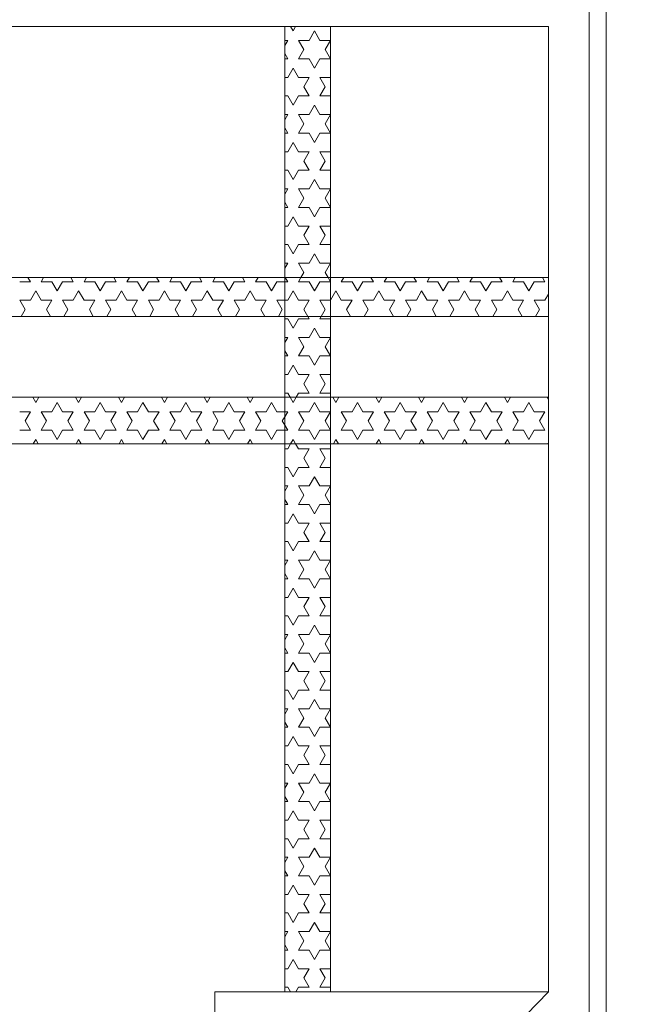
# Model space of a CAD drawing. Units: inches. Extents: x 1291 to 2095, y 532 to 1090.
# Tile 7 of 14: x 1640 to 1663, y 761 to 798. Entities that reach past the tile are written whole.
import ezdxf

# ---------------------------------------------------------------- set-up
doc = ezdxf.new("R2010")
doc.units = ezdxf.units.IN
doc.header["$MEASUREMENT"] = 0
doc.layers.add('A-ANNO-DIMS', color=2, linetype='Continuous', lineweight=18)
doc.layers.add('A-FURN', color=8, linetype='Continuous', lineweight=18)
doc.styles.get("Standard").update_dxf_attribs({"font": 'arial.ttf'})
doc.dimstyles.get("Standard").update_dxf_attribs({"dimtxt": 4, "dimasz": 0.18, "dimexe": 0.18, "dimexo": 0.0625, "dimgap": 0.09, "dimtad": 0, "dimtih": 1, "dimtoh": 1, "dimdec": 0, "dimrnd": 6, "dimzin": 0, "dimdsep": 46, "dimlunit": 3, "dimtxsty": 'Standard', "dimcen": 0.09, "dimadec": 0, "dimazin": 0, "dimtfac": 1, "dimtdec": 0, "dimtofl": 0, "dimtmove": 0, "dimatfit": 3, "dimfxl": 1, "dimtolj": 1, "dimtzin": 0, "dimarcsym": 0})

# ---------------------------------------------------------------- blocks, each defined once
blk = doc.blocks.new('A$C73B76B3A')
for p, q in [((0, 0), (0, 2)), ((0.02, 0.02), (0.02, 1.98)), ((0.4562, 1.5889), (0.0673, 1.1899)), ((0.4562, 1.5889), (0.4562, 1.1899)), ((0.4562, 1.1899), (0.0673, 1.1899)), ((0.0673, 1.1899), (0.0673, 0.0644)), ((0.3214, 1.1899), (0.3214, 0.0644)), ((0.3214, 1.1845), (0.3339, 1.1845)), ((0.3277, 1.1737), (0.3339, 1.1845)), ((0.3464, 1.1845), (0.3589, 1.1845)), ((0.3527, 1.1737), (0.3464, 1.1845)), ((0.3589, 1.1845), (0.362, 1.1899)), ((0.3714, 1.1845), (0.3683, 1.1899)), ((0.3714, 1.1845), (0.3749, 1.1845)), ((0.3749, 1.1899), (0.3749, 0.0644)), ((0.3339, 1.1629), (0.3277, 1.1737)), ((0.3464, 1.1629), (0.3527, 1.1737)), ((0.3214, 1.1629), (0.3339, 1.1629)), ((0.3464, 1.1629), (0.3589, 1.1629)), ((0.3652, 1.1521), (0.3589, 1.1629)), ((0.3652, 1.1521), (0.3714, 1.1629)), ((0.3714, 1.1629), (0.3749, 1.1629)), ((0.3339, 1.1412), (0.3402, 1.1521)), ((0.3464, 1.1412), (0.3402, 1.1521)), ((0.3214, 1.1412), (0.3339, 1.1412)), ((0.3277, 1.1304), (0.3214, 1.1412)), ((0.3464, 1.1412), (0.3589, 1.1412)), ((0.3527, 1.1304), (0.3589, 1.1412)), ((0.3714, 1.1412), (0.3749, 1.1412)), ((0.3749, 1.1352), (0.3714, 1.1412)), ((0.3214, 1.1196), (0.3277, 1.1304)), ((0.3589, 1.1196), (0.3527, 1.1304)), ((0.3714, 1.1196), (0.3749, 1.1257)), ((0.3214, 1.1196), (0.3339, 1.1196)), ((0.3402, 1.1088), (0.3339, 1.1196)), ((0.3402, 1.1088), (0.3464, 1.1196)), ((0.3464, 1.1196), (0.3589, 1.1196)), ((0.3714, 1.1196), (0.3749, 1.1196)), ((0.3589, 1.0979), (0.3652, 1.1088)), ((0.3714, 1.0979), (0.3652, 1.1088)), ((0.3214, 1.0979), (0.3339, 1.0979)), ((0.3277, 1.0871), (0.3339, 1.0979)), ((0.3464, 1.0979), (0.3589, 1.0979)), ((0.3527, 1.0871), (0.3464, 1.0979)), ((0.3714, 1.0979), (0.3749, 1.0979)), ((0.3339, 1.0763), (0.3277, 1.0871)), ((0.3464, 1.0763), (0.3527, 1.0871)), ((0.3214, 1.0763), (0.3339, 1.0763)), ((0.3464, 1.0763), (0.3589, 1.0763)), ((0.3652, 1.0655), (0.3589, 1.0763)), ((0.3652, 1.0655), (0.3714, 1.0763)), ((0.3714, 1.0763), (0.3749, 1.0763)), ((0.3339, 1.0546), (0.3402, 1.0655)), ((0.3464, 1.0546), (0.3402, 1.0655)), ((0.3214, 1.0546), (0.3339, 1.0546)), ((0.3277, 1.0438), (0.3214, 1.0546)), ((0.3464, 1.0546), (0.3589, 1.0546)), ((0.3527, 1.0438), (0.3589, 1.0546)), ((0.3714, 1.0546), (0.3749, 1.0546)), ((0.3749, 1.0486), (0.3714, 1.0546)), ((0.3214, 1.033), (0.3277, 1.0438)), ((0.3589, 1.033), (0.3527, 1.0438)), ((0.3714, 1.033), (0.3749, 1.0391)), ((0.3214, 1.033), (0.3339, 1.033)), ((0.3402, 1.0222), (0.3339, 1.033)), ((0.3402, 1.0222), (0.3464, 1.033)), ((0.3464, 1.033), (0.3589, 1.033)), ((0.3589, 1.0113), (0.3652, 1.0222)), ((0.3714, 1.0113), (0.3652, 1.0222)), ((0.3714, 1.033), (0.3749, 1.033)), ((0.3214, 1.0113), (0.3339, 1.0113)), ((0.3277, 1.0005), (0.3339, 1.0113)), ((0.3464, 1.0113), (0.3589, 1.0113)), ((0.3527, 1.0005), (0.3464, 1.0113)), ((0.3714, 1.0113), (0.3749, 1.0113)), ((0.3339, 0.9897), (0.3277, 1.0005)), ((0.3464, 0.9897), (0.3527, 1.0005)), ((0.3214, 0.9897), (0.3339, 0.9897)), ((0.3464, 0.9897), (0.3589, 0.9897)), ((0.3652, 0.9789), (0.3589, 0.9897)), ((0.3652, 0.9789), (0.3714, 0.9897)), ((0.3714, 0.9897), (0.3749, 0.9897)), ((0.3339, 0.968), (0.3402, 0.9789)), ((0.3464, 0.968), (0.3402, 0.9789)), ((0.3214, 0.968), (0.3339, 0.968)), ((0.3277, 0.9572), (0.3214, 0.968)), ((0.3464, 0.968), (0.3589, 0.968)), ((0.3527, 0.9572), (0.3589, 0.968)), ((0.3714, 0.968), (0.3749, 0.968)), ((0.3749, 0.962), (0.3714, 0.968)), ((0.3214, 0.9464), (0.3277, 0.9572)), ((0.3589, 0.9464), (0.3527, 0.9572)), ((0.3214, 0.9464), (0.3339, 0.9464)), ((0.3402, 0.9356), (0.3339, 0.9464)), ((0.3402, 0.9356), (0.3464, 0.9464)), ((0.3464, 0.9464), (0.3589, 0.9464)), ((0.3714, 0.9464), (0.3749, 0.9525)), ((0.3714, 0.9464), (0.3749, 0.9464)), ((0.3589, 0.9247), (0.3652, 0.9356)), ((0.3714, 0.9247), (0.3652, 0.9356)), ((0.3214, 0.9247), (0.3339, 0.9247)), ((0.3277, 0.9139), (0.3339, 0.9247)), ((0.3464, 0.9247), (0.3589, 0.9247)), ((0.3527, 0.9139), (0.3464, 0.9247)), ((0.3714, 0.9247), (0.3749, 0.9247)), ((0.3339, 0.9031), (0.3277, 0.9139)), ((0.3464, 0.9031), (0.3527, 0.9139)), ((0.3214, 0.9031), (0.3339, 0.9031)), ((0.3464, 0.9031), (0.3589, 0.9031)), ((0.3652, 0.8923), (0.3589, 0.9031)), ((0.3652, 0.8923), (0.3714, 0.9031)), ((0.3714, 0.9031), (0.3749, 0.9031)), ((0.3339, 0.8814), (0.3402, 0.8923)), ((0.3464, 0.8814), (0.3402, 0.8923)), ((0.3214, 0.8814), (0.3339, 0.8814)), ((0.3277, 0.8706), (0.3214, 0.8814)), ((0.3464, 0.8814), (0.3589, 0.8814)), ((0.3527, 0.8706), (0.3589, 0.8814)), ((0.3714, 0.8814), (0.3749, 0.8814)), ((0.3749, 0.8754), (0.3714, 0.8814)), ((0.3214, 0.8598), (0.3277, 0.8706)), ((0.3589, 0.8598), (0.3527, 0.8706)), ((0.3714, 0.8598), (0.3749, 0.8659)), ((0.3214, 0.8598), (0.3339, 0.8598)), ((0.3402, 0.849), (0.3339, 0.8598)), ((0.3402, 0.849), (0.3464, 0.8598)), ((0.3464, 0.8598), (0.3589, 0.8598)), ((0.3714, 0.8598), (0.3749, 0.8598)), ((0.3214, 0.8381), (0.3339, 0.8381)), ((0.3277, 0.8273), (0.3339, 0.8381)), ((0.3464, 0.8381), (0.3589, 0.8381)), ((0.3527, 0.8273), (0.3464, 0.8381)), ((0.3589, 0.8381), (0.3652, 0.849)), ((0.3714, 0.8381), (0.3652, 0.849)), ((0.3714, 0.8381), (0.3749, 0.8381)), ((0.3339, 0.8165), (0.3277, 0.8273)), ((0.3464, 0.8165), (0.3527, 0.8273)), ((0.3214, 0.8165), (0.3339, 0.8165)), ((0.3464, 0.8165), (0.3589, 0.8165)), ((0.3652, 0.8057), (0.3589, 0.8165)), ((0.3652, 0.8057), (0.3714, 0.8165)), ((0.3714, 0.8165), (0.3749, 0.8165)), ((0.3339, 0.7948), (0.3402, 0.8057)), ((0.3464, 0.7948), (0.3402, 0.8057)), ((0.3214, 0.7948), (0.3339, 0.7948)), ((0.3277, 0.784), (0.3214, 0.7948)), ((0.3464, 0.7948), (0.3589, 0.7948)), ((0.3527, 0.784), (0.3589, 0.7948)), ((0.3714, 0.7948), (0.3749, 0.7948)), ((0.3749, 0.7888), (0.3714, 0.7948)), ((0.3214, 0.7732), (0.3277, 0.784)), ((0.3589, 0.7732), (0.3527, 0.784)), ((0.3214, 0.7732), (0.3339, 0.7732)), ((0.3402, 0.7624), (0.3339, 0.7732)), ((0.3402, 0.7624), (0.3464, 0.7732)), ((0.3464, 0.7732), (0.3589, 0.7732)), ((0.3714, 0.7732), (0.3749, 0.7793)), ((0.3714, 0.7732), (0.3749, 0.7732)), ((0.3589, 0.7515), (0.3652, 0.7624)), ((0.3714, 0.7515), (0.3652, 0.7624)), ((0.3214, 0.7515), (0.3339, 0.7515)), ((0.3277, 0.7407), (0.3339, 0.7515)), ((0.3464, 0.7515), (0.3589, 0.7515)), ((0.3527, 0.7407), (0.3464, 0.7515)), ((0.3714, 0.7515), (0.3749, 0.7515)), ((0.3339, 0.7299), (0.3277, 0.7407)), ((0.3464, 0.7299), (0.3527, 0.7407)), ((0.3214, 0.7299), (0.3339, 0.7299)), ((0.3464, 0.7299), (0.3589, 0.7299)), ((0.3652, 0.7191), (0.3589, 0.7299)), ((0.3652, 0.7191), (0.3714, 0.7299)), ((0.3714, 0.7299), (0.3749, 0.7299)), ((0.3339, 0.7082), (0.3402, 0.7191)), ((0.3464, 0.7082), (0.3402, 0.7191)), ((0.3214, 0.7082), (0.3339, 0.7082)), ((0.3277, 0.6974), (0.3214, 0.7082)), ((0.3464, 0.7082), (0.3589, 0.7082)), ((0.3527, 0.6974), (0.3589, 0.7082)), ((0.3714, 0.7082), (0.3749, 0.7082)), ((0.3749, 0.7022), (0.3714, 0.7082)), ((0.3214, 0.6866), (0.3277, 0.6974)), ((0.3589, 0.6866), (0.3527, 0.6974)), ((0.3714, 0.6866), (0.3749, 0.6926)), ((0.3214, 0.6866), (0.3339, 0.6866)), ((0.3402, 0.6758), (0.3339, 0.6866)), ((0.3402, 0.6758), (0.3464, 0.6866)), ((0.3464, 0.6866), (0.3589, 0.6866)), ((0.3714, 0.6866), (0.3749, 0.6866)), ((0.3589, 0.6649), (0.3652, 0.6758)), ((0.3714, 0.6649), (0.3652, 0.6758)), ((0.3214, 0.6649), (0.3339, 0.6649)), ((0.3277, 0.6541), (0.3339, 0.6649)), ((0.3464, 0.6649), (0.3589, 0.6649)), ((0.3527, 0.6541), (0.3464, 0.6649)), ((0.3714, 0.6649), (0.3749, 0.6649)), ((0.3214, 0.6433), (0.3339, 0.6433)), ((0.3339, 0.6433), (0.3277, 0.6541)), ((0.3464, 0.6433), (0.3527, 0.6541)), ((0.3464, 0.6433), (0.3589, 0.6433)), ((0.3652, 0.6325), (0.3589, 0.6433)), ((0.3652, 0.6325), (0.3714, 0.6433)), ((0.3714, 0.6433), (0.3749, 0.6433)), ((0.3339, 0.6216), (0.3402, 0.6325)), ((0.3464, 0.6216), (0.3402, 0.6325)), ((0.3214, 0.6216), (0.3339, 0.6216)), ((0.3277, 0.6108), (0.3214, 0.6216)), ((0.3464, 0.6216), (0.3589, 0.6216)), ((0.3527, 0.6108), (0.3589, 0.6216)), ((0.3714, 0.6216), (0.3749, 0.6216)), ((0.3749, 0.6156), (0.3714, 0.6216)), ((0.3214, 0.6), (0.3277, 0.6108)), ((0.3589, 0.6), (0.3527, 0.6108)), ((0.3214, 0.6), (0.3339, 0.6)), ((0.3402, 0.5892), (0.3339, 0.6)), ((0.3402, 0.5892), (0.3464, 0.6)), ((0.3464, 0.6), (0.3589, 0.6)), ((0.3714, 0.6), (0.3749, 0.606)), ((0.3714, 0.6), (0.3749, 0.6)), ((0.3589, 0.5783), (0.3652, 0.5892)), ((0.3714, 0.5783), (0.3652, 0.5892)), ((0.3214, 0.5783), (0.3339, 0.5783)), ((0.3277, 0.5675), (0.3339, 0.5783)), ((0.3464, 0.5783), (0.3589, 0.5783)), ((0.3527, 0.5675), (0.3464, 0.5783)), ((0.3714, 0.5783), (0.3749, 0.5783)), ((0.3339, 0.5567), (0.3277, 0.5675)), ((0.3464, 0.5567), (0.3527, 0.5675)), ((0.3214, 0.5567), (0.3339, 0.5567)), ((0.3464, 0.5567), (0.3589, 0.5567)), ((0.3623, 0.5509), (0.3589, 0.5567)), ((0.3681, 0.5509), (0.3714, 0.5567)), ((0.3714, 0.5567), (0.3749, 0.5567)), ((1.2954, 0.5509), (0.0673, 0.5509)), ((0.0673, 0.5495), (0.0681, 0.5509)), ((0.0839, 0.535), (0.0902, 0.5459)), ((0.0964, 0.535), (0.0902, 0.5459)), ((0.1152, 0.5459), (0.1123, 0.5509)), ((0.1152, 0.5459), (0.1181, 0.5509)), ((0.1339, 0.535), (0.1402, 0.5459)), ((0.1464, 0.535), (0.1402, 0.5459)), ((0.1652, 0.5459), (0.1623, 0.5509)), ((0.1652, 0.5459), (0.1681, 0.5509)), ((0.1839, 0.535), (0.1902, 0.5459)), ((0.1964, 0.535), (0.1902, 0.5459)), ((0.2152, 0.5459), (0.2123, 0.5509)), ((0.2152, 0.5459), (0.2181, 0.5509)), ((0.2339, 0.535), (0.2402, 0.5459)), ((0.2464, 0.535), (0.2402, 0.5459)), ((0.2652, 0.5459), (0.2623, 0.5509)), ((0.2652, 0.5459), (0.2681, 0.5509)), ((0.2839, 0.535), (0.2902, 0.5459)), ((0.2964, 0.535), (0.2902, 0.5459)), ((0.3152, 0.5459), (0.3123, 0.5509)), ((0.3152, 0.5459), (0.3181, 0.5509)), ((0.3339, 0.535), (0.3402, 0.5459)), ((0.3464, 0.535), (0.3402, 0.5459)), ((0.3652, 0.5459), (0.3623, 0.5509)), ((0.3652, 0.5459), (0.3681, 0.5509)), ((0.3839, 0.535), (0.3902, 0.5459)), ((0.3964, 0.535), (0.3902, 0.5459)), ((0.4152, 0.5459), (0.4123, 0.5509)), ((0.4152, 0.5459), (0.4181, 0.5509)), ((0.4339, 0.535), (0.4402, 0.5459)), ((0.4464, 0.535), (0.4402, 0.5459)), ((0.4652, 0.5459), (0.4623, 0.5509)), ((0.4652, 0.5459), (0.4681, 0.5509)), ((0.4839, 0.535), (0.4902, 0.5459)), ((0.4964, 0.535), (0.4902, 0.5459)), ((0.5152, 0.5459), (0.5123, 0.5509)), ((0.5152, 0.5459), (0.5181, 0.5509)), ((0.5339, 0.535), (0.5402, 0.5459)), ((0.5464, 0.535), (0.5402, 0.5459)), ((0.5652, 0.5459), (0.5623, 0.5509)), ((0.5652, 0.5459), (0.5681, 0.5509)), ((0.5839, 0.535), (0.5902, 0.5459)), ((0.5964, 0.535), (0.5902, 0.5459)), ((0.6152, 0.5459), (0.6123, 0.5509)), ((0.6152, 0.5459), (0.6181, 0.5509)), ((0.6339, 0.535), (0.6402, 0.5459)), ((0.6464, 0.535), (0.6402, 0.5459)), ((0.6652, 0.5459), (0.6623, 0.5509)), ((0.6652, 0.5459), (0.6681, 0.5509)), ((0.0714, 0.535), (0.0839, 0.535)), ((0.0777, 0.5242), (0.0714, 0.535)), ((0.0964, 0.535), (0.1089, 0.535)), ((0.1027, 0.5242), (0.1089, 0.535)), ((0.1214, 0.535), (0.1339, 0.535)), ((0.1277, 0.5242), (0.1214, 0.535)), ((0.1464, 0.535), (0.1589, 0.535)), ((0.1527, 0.5242), (0.1589, 0.535)), ((0.1714, 0.535), (0.1839, 0.535)), ((0.1777, 0.5242), (0.1714, 0.535)), ((0.1964, 0.535), (0.2089, 0.535)), ((0.2027, 0.5242), (0.2089, 0.535)), ((0.2214, 0.535), (0.2339, 0.535)), ((0.2277, 0.5242), (0.2214, 0.535)), ((0.2464, 0.535), (0.2589, 0.535)), ((0.2527, 0.5242), (0.2589, 0.535)), ((0.2714, 0.535), (0.2839, 0.535)), ((0.2777, 0.5242), (0.2714, 0.535)), ((0.2964, 0.535), (0.3089, 0.535)), ((0.3027, 0.5242), (0.3089, 0.535)), ((0.3214, 0.535), (0.3214, 0.535)), ((0.3214, 0.535), (0.3339, 0.535)), ((0.3214, 0.535), (0.3214, 0.535)), ((0.3277, 0.5242), (0.3214, 0.535)), ((0.3464, 0.535), (0.3589, 0.535)), ((0.3527, 0.5242), (0.3589, 0.535)), ((0.3714, 0.535), (0.3749, 0.535)), ((0.3749, 0.529), (0.3714, 0.535)), ((0.3749, 0.535), (0.3839, 0.535)), ((0.3777, 0.5242), (0.3749, 0.529)), ((0.3964, 0.535), (0.4089, 0.535)), ((0.4027, 0.5242), (0.4089, 0.535)), ((0.4214, 0.535), (0.4339, 0.535)), ((0.4277, 0.5242), (0.4214, 0.535)), ((0.4464, 0.535), (0.4589, 0.535)), ((0.4527, 0.5242), (0.4589, 0.535)), ((0.4714, 0.535), (0.4839, 0.535)), ((0.4777, 0.5242), (0.4714, 0.535)), ((0.4964, 0.535), (0.5089, 0.535)), ((0.5027, 0.5242), (0.5089, 0.535)), ((0.5214, 0.535), (0.5339, 0.535)), ((0.5277, 0.5242), (0.5214, 0.535)), ((0.5464, 0.535), (0.5589, 0.535)), ((0.5527, 0.5242), (0.5589, 0.535)), ((0.5714, 0.535), (0.5839, 0.535)), ((0.5777, 0.5242), (0.5714, 0.535)), ((0.5964, 0.535), (0.6089, 0.535)), ((0.6027, 0.5242), (0.6089, 0.535)), ((0.6214, 0.535), (0.6339, 0.535)), ((0.6277, 0.5242), (0.6214, 0.535)), ((0.6464, 0.535), (0.6589, 0.535)), ((0.6527, 0.5242), (0.6589, 0.535)), ((0.6714, 0.535), (0.6839, 0.535)), ((0.6777, 0.5242), (0.6714, 0.535)), ((0.0714, 0.5134), (0.0777, 0.5242)), ((0.1089, 0.5134), (0.1027, 0.5242)), ((0.1214, 0.5134), (0.1277, 0.5242)), ((0.1589, 0.5134), (0.1527, 0.5242)), ((0.1714, 0.5134), (0.1777, 0.5242)), ((0.2089, 0.5134), (0.2027, 0.5242)), ((0.2214, 0.5134), (0.2277, 0.5242)), ((0.2589, 0.5134), (0.2527, 0.5242)), ((0.2714, 0.5134), (0.2777, 0.5242)), ((0.3089, 0.5134), (0.3027, 0.5242)), ((0.3214, 0.5134), (0.3277, 0.5242)), ((0.3589, 0.5134), (0.3527, 0.5242)), ((0.3714, 0.5134), (0.3749, 0.5194)), ((0.3749, 0.5194), (0.3777, 0.5242)), ((0.4089, 0.5134), (0.4027, 0.5242)), ((0.4214, 0.5134), (0.4277, 0.5242)), ((0.4589, 0.5134), (0.4527, 0.5242)), ((0.4714, 0.5134), (0.4777, 0.5242)), ((0.5089, 0.5134), (0.5027, 0.5242)), ((0.5214, 0.5134), (0.5277, 0.5242)), ((0.5589, 0.5134), (0.5527, 0.5242)), ((0.5714, 0.5134), (0.5777, 0.5242)), ((0.6089, 0.5134), (0.6027, 0.5242)), ((0.6214, 0.5134), (0.6277, 0.5242)), ((0.6589, 0.5134), (0.6527, 0.5242)), ((0.6714, 0.5134), (0.6777, 0.5242)), ((0.0714, 0.5134), (0.0839, 0.5134)), ((0.0902, 0.5026), (0.0839, 0.5134)), ((0.0902, 0.5026), (0.0964, 0.5134)), ((0.0964, 0.5134), (0.1089, 0.5134)), ((0.1214, 0.5134), (0.1339, 0.5134)), ((0.1402, 0.5026), (0.1339, 0.5134)), ((0.1402, 0.5026), (0.1464, 0.5134)), ((0.1464, 0.5134), (0.1589, 0.5134)), ((0.1714, 0.5134), (0.1839, 0.5134)), ((0.1902, 0.5026), (0.1839, 0.5134)), ((0.1902, 0.5026), (0.1964, 0.5134)), ((0.1964, 0.5134), (0.2089, 0.5134)), ((0.2214, 0.5134), (0.2339, 0.5134)), ((0.2402, 0.5026), (0.2339, 0.5134)), ((0.2402, 0.5026), (0.2464, 0.5134)), ((0.2464, 0.5134), (0.2589, 0.5134)), ((0.2714, 0.5134), (0.2839, 0.5134)), ((0.2902, 0.5026), (0.2839, 0.5134)), ((0.2902, 0.5026), (0.2964, 0.5134)), ((0.2964, 0.5134), (0.3089, 0.5134)), ((0.3214, 0.5134), (0.3214, 0.5134)), ((0.3214, 0.5134), (0.3339, 0.5134)), ((0.3214, 0.5134), (0.3214, 0.5134)), ((0.3402, 0.5026), (0.3339, 0.5134)), ((0.3402, 0.5026), (0.3464, 0.5134)), ((0.3464, 0.5134), (0.3589, 0.5134)), ((0.3714, 0.5134), (0.3749, 0.5134)), ((0.3749, 0.5134), (0.3839, 0.5134)), ((0.3902, 0.5026), (0.3839, 0.5134)), ((0.3902, 0.5026), (0.3964, 0.5134)), ((0.3964, 0.5134), (0.4089, 0.5134)), ((0.4214, 0.5134), (0.4339, 0.5134)), ((0.4402, 0.5026), (0.4339, 0.5134)), ((0.4402, 0.5026), (0.4464, 0.5134)), ((0.4464, 0.5134), (0.4589, 0.5134)), ((0.4714, 0.5134), (0.4839, 0.5134)), ((0.4902, 0.5026), (0.4839, 0.5134)), ((0.4902, 0.5026), (0.4964, 0.5134)), ((0.4964, 0.5134), (0.5089, 0.5134)), ((0.5214, 0.5134), (0.5339, 0.5134)), ((0.5402, 0.5026), (0.5339, 0.5134)), ((0.5402, 0.5026), (0.5464, 0.5134)), ((0.5464, 0.5134), (0.5589, 0.5134)), ((0.5714, 0.5134), (0.5839, 0.5134)), ((0.5902, 0.5026), (0.5839, 0.5134)), ((0.5902, 0.5026), (0.5964, 0.5134)), ((0.5964, 0.5134), (0.6089, 0.5134)), ((0.6214, 0.5134), (0.6339, 0.5134)), ((0.6402, 0.5026), (0.6339, 0.5134)), ((0.6402, 0.5026), (0.6464, 0.5134)), ((0.6464, 0.5134), (0.6589, 0.5134)), ((0.6714, 0.5134), (0.6839, 0.5134)), ((0.0687, 0.4965), (0.0673, 0.4989)), ((1.2954, 0.4965), (0.0673, 0.4965)), ((0.1117, 0.4965), (0.1152, 0.5026)), ((0.1187, 0.4965), (0.1152, 0.5026)), ((0.1617, 0.4965), (0.1652, 0.5026)), ((0.1687, 0.4965), (0.1652, 0.5026)), ((0.2117, 0.4965), (0.2152, 0.5026)), ((0.2187, 0.4965), (0.2152, 0.5026)), ((0.2617, 0.4965), (0.2652, 0.5026)), ((0.2687, 0.4965), (0.2652, 0.5026)), ((0.3117, 0.4965), (0.3152, 0.5026)), ((0.3187, 0.4965), (0.3152, 0.5026)), ((0.3589, 0.4917), (0.3617, 0.4965)), ((0.3617, 0.4965), (0.3652, 0.5026)), ((0.3687, 0.4965), (0.3652, 0.5026)), ((0.3714, 0.4917), (0.3687, 0.4965)), ((0.4117, 0.4965), (0.4152, 0.5026)), ((0.4187, 0.4965), (0.4152, 0.5026)), ((0.4617, 0.4965), (0.4652, 0.5026)), ((0.4687, 0.4965), (0.4652, 0.5026)), ((0.5117, 0.4965), (0.5152, 0.5026)), ((0.5187, 0.4965), (0.5152, 0.5026)), ((0.5617, 0.4965), (0.5652, 0.5026)), ((0.5687, 0.4965), (0.5652, 0.5026)), ((0.6117, 0.4965), (0.6152, 0.5026)), ((0.6187, 0.4965), (0.6152, 0.5026)), ((0.6617, 0.4965), (0.6652, 0.5026)), ((0.6687, 0.4965), (0.6652, 0.5026)), ((0.3214, 0.4917), (0.3339, 0.4917)), ((0.3277, 0.4809), (0.3339, 0.4917)), ((0.3464, 0.4917), (0.3589, 0.4917)), ((0.3527, 0.4809), (0.3464, 0.4917)), ((0.3714, 0.4917), (0.3749, 0.4917)), ((0.3339, 0.4701), (0.3277, 0.4809)), ((0.3464, 0.4701), (0.3527, 0.4809)), ((0.3214, 0.4701), (0.3339, 0.4701)), ((0.3339, 0.4484), (0.3402, 0.4593)), ((0.3464, 0.4484), (0.3402, 0.4593)), ((0.3464, 0.4701), (0.3589, 0.4701)), ((0.3652, 0.4593), (0.3589, 0.4701)), ((0.3652, 0.4593), (0.3714, 0.4701)), ((0.3714, 0.4701), (0.3749, 0.4701)), ((0.3214, 0.4484), (0.3339, 0.4484)), ((0.3277, 0.4376), (0.3214, 0.4484)), ((0.3464, 0.4484), (0.3589, 0.4484)), ((0.3527, 0.4376), (0.3589, 0.4484)), ((0.3714, 0.4484), (0.3749, 0.4484)), ((0.3749, 0.4424), (0.3714, 0.4484)), ((0.3214, 0.4268), (0.3277, 0.4376)), ((0.3589, 0.4268), (0.3527, 0.4376)), ((0.3214, 0.4268), (0.3339, 0.4268)), ((0.3402, 0.4159), (0.3339, 0.4268)), ((0.3402, 0.4159), (0.3464, 0.4268)), ((0.3464, 0.4268), (0.3589, 0.4268)), ((0.3714, 0.4268), (0.3749, 0.4328)), ((0.3714, 0.4268), (0.3749, 0.4268)), ((0.3589, 0.4051), (0.3652, 0.4159)), ((0.3714, 0.4051), (0.3652, 0.4159)), ((1.2954, 0.4023), (0.0673, 0.4023)), ((0.0777, 0.3943), (0.0823, 0.4023)), ((0.1027, 0.3943), (0.0981, 0.4023)), ((0.1277, 0.3943), (0.1323, 0.4023)), ((0.1527, 0.3943), (0.1481, 0.4023)), ((0.1777, 0.3943), (0.1823, 0.4023)), ((0.2027, 0.3943), (0.1981, 0.4023)), ((0.2277, 0.3943), (0.2323, 0.4023)), ((0.2527, 0.3943), (0.2481, 0.4023)), ((0.2777, 0.3943), (0.2823, 0.4023)), ((0.3027, 0.3943), (0.2981, 0.4023)), ((0.3214, 0.4051), (0.3339, 0.4051)), ((0.3277, 0.3943), (0.3323, 0.4023)), ((0.3323, 0.4023), (0.3339, 0.4051)), ((0.3464, 0.4051), (0.3589, 0.4051)), ((0.3481, 0.4023), (0.3464, 0.4051)), ((0.3527, 0.3943), (0.3481, 0.4023)), ((0.3714, 0.4051), (0.3749, 0.4051)), ((0.3777, 0.3943), (0.3823, 0.4023)), ((0.4027, 0.3943), (0.3981, 0.4023)), ((0.4277, 0.3943), (0.4323, 0.4023)), ((0.4527, 0.3943), (0.4481, 0.4023)), ((0.4777, 0.3943), (0.4823, 0.4023)), ((0.5027, 0.3943), (0.4981, 0.4023)), ((0.5277, 0.3943), (0.5323, 0.4023)), ((0.5527, 0.3943), (0.5481, 0.4023)), ((0.5777, 0.3943), (0.5823, 0.4023)), ((0.6027, 0.3943), (0.5981, 0.4023)), ((0.6277, 0.3943), (0.6323, 0.4023)), ((0.6527, 0.3943), (0.6481, 0.4023)), ((0.6777, 0.3943), (0.6823, 0.4023)), ((0.0839, 0.3835), (0.0777, 0.3943)), ((0.0964, 0.3835), (0.1027, 0.3943)), ((0.1339, 0.3835), (0.1277, 0.3943)), ((0.1464, 0.3835), (0.1527, 0.3943)), ((0.1839, 0.3835), (0.1777, 0.3943)), ((0.1964, 0.3835), (0.2027, 0.3943)), ((0.2339, 0.3835), (0.2277, 0.3943)), ((0.2464, 0.3835), (0.2527, 0.3943)), ((0.2839, 0.3835), (0.2777, 0.3943)), ((0.2964, 0.3835), (0.3027, 0.3943)), ((0.3339, 0.3835), (0.3277, 0.3943)), ((0.3464, 0.3835), (0.3527, 0.3943)), ((0.3839, 0.3835), (0.3777, 0.3943)), ((0.3964, 0.3835), (0.4027, 0.3943)), ((0.4339, 0.3835), (0.4277, 0.3943)), ((0.4464, 0.3835), (0.4527, 0.3943)), ((0.4839, 0.3835), (0.4777, 0.3943)), ((0.4964, 0.3835), (0.5027, 0.3943)), ((0.5339, 0.3835), (0.5277, 0.3943)), ((0.5464, 0.3835), (0.5527, 0.3943)), ((0.5839, 0.3835), (0.5777, 0.3943)), ((0.5964, 0.3835), (0.6027, 0.3943)), ((0.6339, 0.3835), (0.6277, 0.3943)), ((0.6464, 0.3835), (0.6527, 0.3943)), ((0.6839, 0.3835), (0.6777, 0.3943)), ((0.0673, 0.3763), (0.0714, 0.3835)), ((0.0714, 0.3835), (0.0839, 0.3835)), ((0.0964, 0.3835), (0.1089, 0.3835)), ((0.1152, 0.3726), (0.1089, 0.3835)), ((0.1152, 0.3726), (0.1214, 0.3835)), ((0.1214, 0.3835), (0.1339, 0.3835)), ((0.1464, 0.3835), (0.1589, 0.3835)), ((0.1652, 0.3726), (0.1589, 0.3835)), ((0.1652, 0.3726), (0.1714, 0.3835)), ((0.1714, 0.3835), (0.1839, 0.3835)), ((0.1964, 0.3835), (0.2089, 0.3835)), ((0.2152, 0.3726), (0.2089, 0.3835)), ((0.2152, 0.3726), (0.2214, 0.3835)), ((0.2214, 0.3835), (0.2339, 0.3835)), ((0.2464, 0.3835), (0.2589, 0.3835)), ((0.2652, 0.3726), (0.2589, 0.3835)), ((0.2652, 0.3726), (0.2714, 0.3835)), ((0.2714, 0.3835), (0.2839, 0.3835)), ((0.2964, 0.3835), (0.3089, 0.3835)), ((0.3152, 0.3726), (0.3089, 0.3835)), ((0.3152, 0.3726), (0.3214, 0.3835)), ((0.3214, 0.3835), (0.3214, 0.3835)), ((0.3214, 0.3835), (0.3339, 0.3835)), ((0.3464, 0.3835), (0.3589, 0.3835)), ((0.3652, 0.3726), (0.3589, 0.3835)), ((0.3652, 0.3726), (0.3714, 0.3835)), ((0.3714, 0.3835), (0.3749, 0.3835)), ((0.3749, 0.3835), (0.3839, 0.3835)), ((0.3964, 0.3835), (0.4089, 0.3835)), ((0.4152, 0.3726), (0.4089, 0.3835)), ((0.4152, 0.3726), (0.4214, 0.3835)), ((0.4214, 0.3835), (0.4339, 0.3835)), ((0.4464, 0.3835), (0.4589, 0.3835)), ((0.4652, 0.3726), (0.4589, 0.3835)), ((0.4652, 0.3726), (0.4714, 0.3835)), ((0.4714, 0.3835), (0.4839, 0.3835)), ((0.4964, 0.3835), (0.5089, 0.3835)), ((0.5152, 0.3726), (0.5089, 0.3835)), ((0.5152, 0.3726), (0.5214, 0.3835)), ((0.5214, 0.3835), (0.5339, 0.3835)), ((0.5464, 0.3835), (0.5589, 0.3835)), ((0.5652, 0.3726), (0.5589, 0.3835)), ((0.5652, 0.3726), (0.5714, 0.3835)), ((0.5714, 0.3835), (0.5839, 0.3835)), ((0.5964, 0.3835), (0.6089, 0.3835)), ((0.6152, 0.3726), (0.6089, 0.3835)), ((0.6152, 0.3726), (0.6214, 0.3835)), ((0.6214, 0.3835), (0.6339, 0.3835)), ((0.6464, 0.3835), (0.6589, 0.3835)), ((0.6652, 0.3726), (0.6589, 0.3835)), ((0.6652, 0.3726), (0.6714, 0.3835)), ((0.6714, 0.3835), (0.6839, 0.3835)), ((0.0839, 0.3618), (0.0902, 0.3726)), ((0.0964, 0.3618), (0.0902, 0.3726)), ((0.1339, 0.3618), (0.1402, 0.3726)), ((0.1464, 0.3618), (0.1402, 0.3726)), ((0.1839, 0.3618), (0.1902, 0.3726)), ((0.1964, 0.3618), (0.1902, 0.3726)), ((0.2339, 0.3618), (0.2402, 0.3726)), ((0.2464, 0.3618), (0.2402, 0.3726)), ((0.2839, 0.3618), (0.2902, 0.3726)), ((0.2964, 0.3618), (0.2902, 0.3726)), ((0.3339, 0.3618), (0.3402, 0.3726)), ((0.3464, 0.3618), (0.3402, 0.3726)), ((0.3839, 0.3618), (0.3902, 0.3726)), ((0.3964, 0.3618), (0.3902, 0.3726)), ((0.4339, 0.3618), (0.4402, 0.3726)), ((0.4464, 0.3618), (0.4402, 0.3726)), ((0.4839, 0.3618), (0.4902, 0.3726)), ((0.4964, 0.3618), (0.4902, 0.3726)), ((0.5339, 0.3618), (0.5402, 0.3726)), ((0.5464, 0.3618), (0.5402, 0.3726)), ((0.5839, 0.3618), (0.5902, 0.3726)), ((0.5964, 0.3618), (0.5902, 0.3726)), ((0.6339, 0.3618), (0.6402, 0.3726)), ((0.6464, 0.3618), (0.6402, 0.3726)), ((1.2954, 0.3568), (0.0673, 0.3568)), ((0.0714, 0.3618), (0.0839, 0.3618)), ((0.0743, 0.3568), (0.0714, 0.3618)), ((0.0964, 0.3618), (0.1089, 0.3618)), ((0.106, 0.3568), (0.1089, 0.3618)), ((0.1214, 0.3618), (0.1339, 0.3618)), ((0.1243, 0.3568), (0.1214, 0.3618)), ((0.1464, 0.3618), (0.1589, 0.3618)), ((0.156, 0.3568), (0.1589, 0.3618)), ((0.1714, 0.3618), (0.1839, 0.3618)), ((0.1743, 0.3568), (0.1714, 0.3618)), ((0.1964, 0.3618), (0.2089, 0.3618)), ((0.206, 0.3568), (0.2089, 0.3618)), ((0.2214, 0.3618), (0.2339, 0.3618)), ((0.2243, 0.3568), (0.2214, 0.3618)), ((0.2464, 0.3618), (0.2589, 0.3618)), ((0.256, 0.3568), (0.2589, 0.3618)), ((0.2714, 0.3618), (0.2839, 0.3618)), ((0.2743, 0.3568), (0.2714, 0.3618)), ((0.2964, 0.3618), (0.3089, 0.3618)), ((0.306, 0.3568), (0.3089, 0.3618)), ((0.3214, 0.3618), (0.3214, 0.3618)), ((0.3214, 0.3618), (0.3339, 0.3618)), ((0.3243, 0.3568), (0.3214, 0.3618)), ((0.3214, 0.3618), (0.3214, 0.3618)), ((0.3277, 0.351), (0.3243, 0.3568)), ((0.3464, 0.3618), (0.3589, 0.3618)), ((0.3527, 0.351), (0.356, 0.3568)), ((0.356, 0.3568), (0.3589, 0.3618)), ((0.3714, 0.3618), (0.3749, 0.3618)), ((0.3743, 0.3568), (0.3714, 0.3618)), ((0.3749, 0.3558), (0.3743, 0.3568)), ((0.3749, 0.3618), (0.3839, 0.3618)), ((0.3964, 0.3618), (0.4089, 0.3618)), ((0.406, 0.3568), (0.4089, 0.3618)), ((0.4214, 0.3618), (0.4339, 0.3618)), ((0.4243, 0.3568), (0.4214, 0.3618)), ((0.4464, 0.3618), (0.4589, 0.3618)), ((0.456, 0.3568), (0.4589, 0.3618)), ((0.4714, 0.3618), (0.4839, 0.3618)), ((0.4743, 0.3568), (0.4714, 0.3618)), ((0.4964, 0.3618), (0.5089, 0.3618)), ((0.506, 0.3568), (0.5089, 0.3618)), ((0.5214, 0.3618), (0.5339, 0.3618)), ((0.5243, 0.3568), (0.5214, 0.3618)), ((0.5464, 0.3618), (0.5589, 0.3618)), ((0.556, 0.3568), (0.5589, 0.3618)), ((0.5714, 0.3618), (0.5839, 0.3618)), ((0.5743, 0.3568), (0.5714, 0.3618)), ((0.5964, 0.3618), (0.6089, 0.3618)), ((0.606, 0.3568), (0.6089, 0.3618)), ((0.6214, 0.3618), (0.6339, 0.3618)), ((0.6243, 0.3568), (0.6214, 0.3618)), ((0.6464, 0.3618), (0.6589, 0.3618)), ((0.656, 0.3568), (0.6589, 0.3618)), ((0.6714, 0.3618), (0.6839, 0.3618)), ((0.6743, 0.3568), (0.6714, 0.3618)), ((0.3214, 0.3402), (0.3277, 0.351)), ((0.3589, 0.3402), (0.3527, 0.351)), ((0.3714, 0.3402), (0.3749, 0.3462)), ((0.3214, 0.3402), (0.3339, 0.3402)), ((0.3402, 0.3293), (0.3339, 0.3402)), ((0.3402, 0.3293), (0.3464, 0.3402)), ((0.3464, 0.3402), (0.3589, 0.3402)), ((0.3714, 0.3402), (0.3749, 0.3402)), ((0.3589, 0.3185), (0.3652, 0.3293)), ((0.3714, 0.3185), (0.3652, 0.3293)), ((0.3214, 0.3185), (0.3339, 0.3185)), ((0.3277, 0.3077), (0.3339, 0.3185)), ((0.3464, 0.3185), (0.3589, 0.3185)), ((0.3527, 0.3077), (0.3464, 0.3185)), ((0.3714, 0.3185), (0.3749, 0.3185)), ((0.3339, 0.2969), (0.3277, 0.3077)), ((0.3464, 0.2969), (0.3527, 0.3077)), ((0.3214, 0.2969), (0.3339, 0.2969)), ((0.3464, 0.2969), (0.3589, 0.2969)), ((0.3652, 0.286), (0.3589, 0.2969)), ((0.3652, 0.286), (0.3714, 0.2969)), ((0.3714, 0.2969), (0.3749, 0.2969)), ((0.3339, 0.2752), (0.3402, 0.286)), ((0.3464, 0.2752), (0.3402, 0.286)), ((0.3214, 0.2752), (0.3339, 0.2752)), ((0.3277, 0.2644), (0.3214, 0.2752)), ((0.3214, 0.2536), (0.3277, 0.2644)), ((0.3464, 0.2752), (0.3589, 0.2752)), ((0.3527, 0.2644), (0.3589, 0.2752)), ((0.3589, 0.2536), (0.3527, 0.2644)), ((0.3714, 0.2752), (0.3749, 0.2752)), ((0.3749, 0.2692), (0.3714, 0.2752)), ((0.3214, 0.2536), (0.3339, 0.2536)), ((0.3402, 0.2427), (0.3339, 0.2536)), ((0.3402, 0.2427), (0.3464, 0.2536)), ((0.3464, 0.2536), (0.3589, 0.2536)), ((0.3714, 0.2536), (0.3749, 0.2596)), ((0.3714, 0.2536), (0.3749, 0.2536)), ((0.3589, 0.2319), (0.3652, 0.2427)), ((0.3714, 0.2319), (0.3652, 0.2427)), ((0.3214, 0.2319), (0.3339, 0.2319)), ((0.3277, 0.2211), (0.3339, 0.2319)), ((0.3464, 0.2319), (0.3589, 0.2319)), ((0.3527, 0.2211), (0.3464, 0.2319)), ((0.3714, 0.2319), (0.3749, 0.2319)), ((0.3339, 0.2103), (0.3277, 0.2211)), ((0.3464, 0.2103), (0.3527, 0.2211)), ((0.3214, 0.2103), (0.3339, 0.2103)), ((0.3464, 0.2103), (0.3589, 0.2103)), ((0.3652, 0.1994), (0.3589, 0.2103)), ((0.3652, 0.1994), (0.3714, 0.2103)), ((0.3714, 0.2103), (0.3749, 0.2103)), ((0.3339, 0.1886), (0.3402, 0.1994)), ((0.3464, 0.1886), (0.3402, 0.1994)), ((0.3214, 0.1886), (0.3339, 0.1886)), ((0.3277, 0.1778), (0.3214, 0.1886)), ((0.3464, 0.1886), (0.3589, 0.1886)), ((0.3527, 0.1778), (0.3589, 0.1886)), ((0.3714, 0.1886), (0.3749, 0.1886)), ((0.3749, 0.1826), (0.3714, 0.1886)), ((0.3214, 0.167), (0.3277, 0.1778)), ((0.3589, 0.167), (0.3527, 0.1778)), ((0.3714, 0.167), (0.3749, 0.173)), ((0.3214, 0.167), (0.3339, 0.167)), ((0.3402, 0.1561), (0.3339, 0.167)), ((0.3402, 0.1561), (0.3464, 0.167)), ((0.3464, 0.167), (0.3589, 0.167)), ((0.3714, 0.167), (0.3749, 0.167)), ((0.3589, 0.1453), (0.3652, 0.1561)), ((0.3714, 0.1453), (0.3652, 0.1561)), ((0.3214, 0.1453), (0.3339, 0.1453)), ((0.3277, 0.1345), (0.3339, 0.1453)), ((0.3464, 0.1453), (0.3589, 0.1453)), ((0.3527, 0.1345), (0.3464, 0.1453)), ((0.3714, 0.1453), (0.3749, 0.1453)), ((0.3339, 0.1237), (0.3277, 0.1345)), ((0.3464, 0.1237), (0.3527, 0.1345)), ((0.3214, 0.1237), (0.3339, 0.1237)), ((0.3464, 0.1237), (0.3589, 0.1237)), ((0.3652, 0.1128), (0.3589, 0.1237)), ((0.3652, 0.1128), (0.3714, 0.1237)), ((0.3714, 0.1237), (0.3749, 0.1237)), ((0.3339, 0.102), (0.3402, 0.1128)), ((0.3464, 0.102), (0.3402, 0.1128)), ((0.3214, 0.102), (0.3339, 0.102)), ((0.3277, 0.0912), (0.3214, 0.102)), ((0.3464, 0.102), (0.3589, 0.102)), ((0.3527, 0.0912), (0.3589, 0.102)), ((0.3714, 0.102), (0.3749, 0.102)), ((0.3749, 0.0959), (0.3714, 0.102)), ((0.3214, 0.0804), (0.3277, 0.0912)), ((0.3214, 0.0804), (0.3339, 0.0804)), ((0.3402, 0.0695), (0.3339, 0.0804)), ((0.3402, 0.0695), (0.3464, 0.0804)), ((0.3464, 0.0804), (0.3589, 0.0804)), ((0.3589, 0.0804), (0.3527, 0.0912)), ((0.3714, 0.0804), (0.3749, 0.0864)), ((0.3714, 0.0804), (0.3749, 0.0804)), ((0.3622, 0.0644), (0.3652, 0.0695)), ((0.3681, 0.0644), (0.3652, 0.0695)), ((0.0673, 0.0644), (1.2954, 0.0644))]:
    blk.add_line(p, q)
blk = doc.blocks.new('*D46')
at = {"layer": 'A-ANNO-DIMS', "color": 0, "lineweight": -2, "transparency": 16777216}
for p, q in [((1600.27, 579.843), (1600.27, 1087.16)), ((1685.584, 579.843), (1685.584, 1087.16)), ((1600.45, 1086.98), (1636.471, 1086.98)), ((1685.404, 1086.98), (1649.383, 1086.98))]:
    blk.add_line(p, q, dxfattribs=at)
at = {"layer": 'A-ANNO-DIMS', "color": 0, "transparency": 16777216}
for points in [[(1600.45, 1087.01), (1600.45, 1086.95), (1600.27, 1086.98)], [(1685.404, 1087.01), (1685.404, 1086.95), (1685.584, 1086.98)]]:
    blk.add_solid(points, dxfattribs=at)
at = {"layer": 'Defpoints', "color": 0, "transparency": 16777216}
for p in [(1685.584, 1086.98), (1600.27, 579.78), (1685.584, 579.78)]:
    blk.add_point(p, dxfattribs=at)
at = {"layer": 'A-ANNO-DIMS', "color": 0, "transparency": 16777216, "insert": (1642.927, 1086.98), "char_height": 4, "attachment_point": 5}
blk.add_mtext('\\A1;85.31', dxfattribs=at)
blk = doc.blocks.new('*D49')
at = {"layer": 'A-ANNO-DIMS', "color": 0, "lineweight": -2, "transparency": 16777216}
for p, q in [((1694.074, 852.718), (1694.074, 534.4)), ((1586.074, 816.718), (1586.074, 534.4)), ((1586.254, 534.58), (1635.749, 534.58)), ((1693.894, 534.58), (1644.398, 534.58))]:
    blk.add_line(p, q, dxfattribs=at)
at = {"layer": 'A-ANNO-DIMS', "color": 0, "transparency": 16777216}
for points in [[(1586.254, 534.61), (1586.254, 534.55), (1586.074, 534.58)], [(1693.894, 534.61), (1693.894, 534.55), (1694.074, 534.58)]]:
    blk.add_solid(points, dxfattribs=at)
at = {"layer": 'Defpoints', "color": 0, "transparency": 16777216}
for p in [(1694.074, 852.78), (1586.074, 816.78), (1694.074, 534.58)]:
    blk.add_point(p, dxfattribs=at)
at = {"layer": 'A-ANNO-DIMS', "color": 0, "transparency": 16777216, "insert": (1640.074, 534.58), "char_height": 4, "attachment_point": 5}
blk.add_mtext('\\A1;108', dxfattribs=at)
blk = doc.blocks.new('*D51')
at = {"layer": 'A-ANNO-DIMS', "color": 0, "lineweight": -2, "transparency": 16777216}
for p, q in [((1820.011, 852.78), (1297.694, 852.78)), ((1297.874, 852.6), (1297.874, 794.913)), ((1297.874, 732.96), (1297.874, 790.648)), ((1811.011, 732.78), (1297.694, 732.78))]:
    blk.add_line(p, q, dxfattribs=at)
at = {"layer": 'A-ANNO-DIMS', "color": 0, "transparency": 16777216}
for points in [[(1297.844, 852.6), (1297.904, 852.6), (1297.874, 852.78)], [(1297.844, 732.96), (1297.904, 732.96), (1297.874, 732.78)]]:
    blk.add_solid(points, dxfattribs=at)
at = {"layer": 'Defpoints', "color": 0, "transparency": 16777216}
for p in [(1297.874, 852.78), (1820.074, 852.78), (1811.074, 732.78)]:
    blk.add_point(p, dxfattribs=at)
at = {"layer": 'A-ANNO-DIMS', "color": 0, "transparency": 16777216, "insert": (1297.874, 792.78), "char_height": 4, "attachment_point": 5}
blk.add_mtext('\\A1;120', dxfattribs=at)

msp = doc.modelspace()

# ---------------------------------------------------------------- block references
at = {"layer": 'A-FURN', "xscale": 32.02427574694497, "yscale": 32.02427574694497, "zscale": 32.02427574694497, "rotation": 180}
msp.add_blockref('A$C73B76B3A', (1662.1648, 799.8143), dxfattribs=at)

# ---------------------------------------------------------------- dimensions: what is measured, and where the dimension line sits
at = {"layer": 'A-ANNO-DIMS'}
for base, p1, p2, override, picture, middle in [((1685.5842, 1086.9804), (1600.2697, 579.7804), (1685.5842, 579.7804), {"dimdec": 2, "dimlfac": 1, "dimrnd": 0, "dimzin": 0, "dimdsep": 46, "dimlunit": 2}, '*D46', (1642.927, 1086.9804)), ((1694.0735, 534.5804), (1586.0735, 816.7804), (1694.0735, 852.7804), {"dimdec": 0, "dimlfac": 1, "dimrnd": 0, "dimzin": 0, "dimdsep": 46, "dimlunit": 2}, '*D49', (1640.0735, 534.5804))]:
    dim = msp.add_linear_dim(base=base, p1=p1, p2=p2, dimstyle='Standard', override=override, dxfattribs=at)
    dim.commit()
    dim.dimension.update_dxf_attribs({"geometry": picture, "text_midpoint": middle})
dim = msp.add_linear_dim(base=(1297.8735, 852.7804), p1=(1811.0735, 732.7804), p2=(1820.0735, 852.7804), angle=90, dimstyle='Standard', override={"dimdec": 0, "dimlfac": 1, "dimrnd": 0, "dimzin": 0, "dimdsep": 46, "dimlunit": 2}, dxfattribs=at)
dim.commit()
dim.dimension.update_dxf_attribs({"geometry": '*D51', "text_midpoint": (1297.8735, 792.7804)})

doc.saveas('drawing.dxf')
